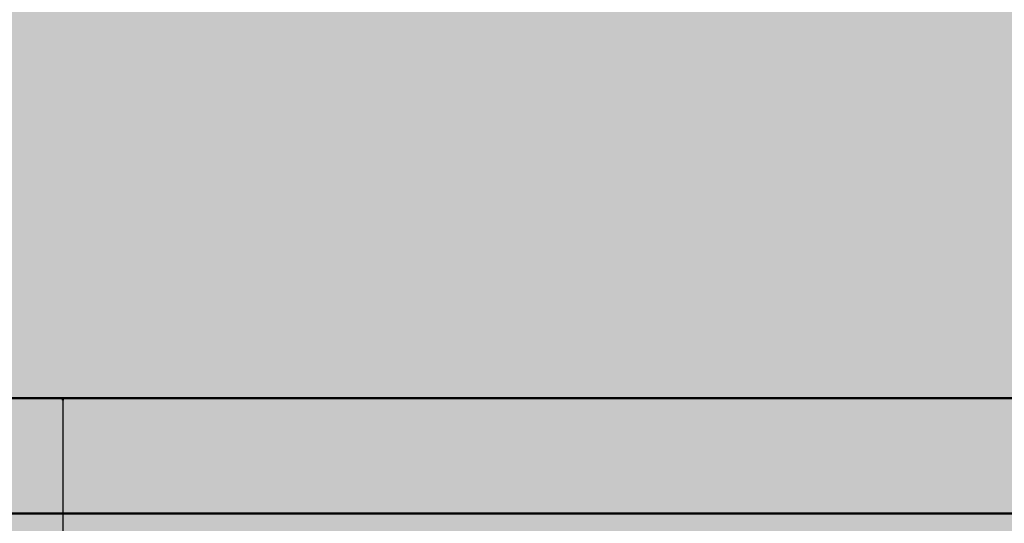
# Model space of a CAD drawing. Units: millimetres. Extents: x 0 to 2267, y 0 to 1823.
# Tile 25 of 256: x 1590 to 1675, y 1117 to 1160. Entities that reach past the tile are written whole.
import ezdxf

# ---------------------------------------------------------------- set-up
doc = ezdxf.new("R2010")
doc.units = ezdxf.units.MM
doc.header["$MEASUREMENT"] = 0
for name, color, linetype, lineweight in [('M-DIMS', 2, 'Continuous', 25), ('M-HATC', 252, 'Continuous', 18), ('M-OUTL', 7, 'Continuous', 50)]:
    doc.layers.add(name, color=color, linetype=linetype, lineweight=lineweight)
doc.styles.get("Standard").update_dxf_attribs({"font": 'arial.ttf'})
doc.dimstyles.get("Standard").update_dxf_attribs({"dimtxt": 7, "dimasz": 4, "dimexe": 0.18, "dimexo": 0.0625, "dimgap": 0.09, "dimtad": 0, "dimdec": 0, "dimzin": 0, "dimdsep": 46, "dimtxsty": 'Standard', "dimcen": 0.09, "dimadec": 0, "dimazin": 0, "dimtfac": 1, "dimtdec": 0, "dimtofl": 0, "dimtmove": 0, "dimatfit": 3, "dimfxl": 1, "dimtolj": 1, "dimtzin": 0, "dimarcsym": 0})

# ---------------------------------------------------------------- blocks, each defined once
blk = doc.blocks.new('*D1')
at = {"layer": 'Defpoints', "color": 0, "transparency": 16777216}
for p in [(1593.429, 1127.417), (1843.429, 1127.417), (1843.429, 955.628)]:
    blk.add_point(p, dxfattribs=at)
at = {"layer": 'M-DIMS', "color": 0, "lineweight": -2, "transparency": 16777216}
for p, q in [((1593.429, 1127.355), (1593.429, 955.448)), ((1843.429, 1127.355), (1843.429, 955.448)), ((1597.429, 955.628), (1710.558, 955.628)), ((1839.429, 955.628), (1726.3, 955.628))]:
    blk.add_line(p, q, dxfattribs=at)
at = {"layer": 'M-DIMS', "color": 0, "transparency": 16777216}
for points in [[(1597.429, 956.294), (1597.429, 954.961), (1593.429, 955.628)], [(1839.429, 956.294), (1839.429, 954.961), (1843.429, 955.628)]]:
    blk.add_solid(points, dxfattribs=at)
at = {"layer": 'M-DIMS', "color": 0, "transparency": 16777216, "insert": (1718.429, 955.628), "char_height": 7, "attachment_point": 5}
blk.add_mtext('\\A1;250', dxfattribs=at)

msp = doc.modelspace()

# ---------------------------------------------------------------- hatches: boundary and pattern name
at = {"layer": 'M-HATC'}
h = msp.add_hatch(color=256, dxfattribs=at)
h.dxf.hatch_style = 1
h.paths.add_polyline_path([(2065.771, 1618.062, 0.236068), (2055.771, 1638.062), (1381.087, 1638.062, 0.236068), (1371.087, 1618.062), (1371.087, 1603.062), (2055.771, 1603.062), (2065.771, 1603.062)])
h.paths.add_polyline_path([(2062.772, 1550.296), (2062.772, 1560.296), (1374.086, 1560.296), (1374.086, 1550.296), (1374.086, 1540.296), (1384.086, 1540.296), (1389.086, 1540.296), (2062.772, 1540.296)])
h.paths.add_polyline_path([(1930.929, 1282.766), (1505.929, 1282.766), (1587.628, 1235.597, 0.131652), (1600.128, 1232.247), (1836.73, 1232.247, 0.131652), (1849.23, 1235.597)])
h.paths.add_polyline_path([(1930.929, 1117.417), (1905.929, 1117.417), (1505.929, 1117.417), (1505.929, 1077.417), (1930.929, 1077.417)])
h = msp.add_hatch(color=256, dxfattribs=at)
h.dxf.hatch_style = 1
h.paths.add_polyline_path([(2055.771, 1603.062), (1381.087, 1603.062), (1381.087, 1598.062), (2055.771, 1598.062)])
h.paths.add_polyline_path([(2055.771, 1598.062), (1381.087, 1598.062), (1381.087, 1593.062), (2055.771, 1593.062)])
h.paths.add_polyline_path([(2051.307, 1536.761), (1385.55, 1536.761), (1385.55, 1526.761), (1387.55, 1526.761), (1388.537, 1525.053), (1385.332, 1521.233), (1385.332, 1521.223), (2050.254, 1522.749), (2048.321, 1525.053), (2049.307, 1526.761), (2051.307, 1526.761)])
edge = h.paths.add_edge_path()
edge.add_arc((1847.535, 1379.149), 135, 222.60306, 222.89085, ccw=False)
edge.add_line((1748.166, 1287.766), (1683.092, 1287.766))
edge.add_arc((1583.724, 1379.149), 135, 317.10915, 317.39694, ccw=False)
edge.add_arc((1678.969, 1290.671), 5, 222.89085, 317.10915, ccw=False)
edge.add_arc((1774.213, 1379.149), 135, 222.60306, 222.89085, ccw=False)
edge.add_line((1674.845, 1287.766), (1609.771, 1287.766))
edge.add_arc((1510.403, 1379.149), 135, 317.10915, 317.39694, ccw=False)
edge.add_arc((1605.647, 1290.671), 5, 222.89085, 317.10915, ccw=False)
edge.add_arc((1700.892, 1379.149), 135, 222.60306, 222.89085, ccw=False)
edge.add_line((1601.524, 1287.766), (1536.45, 1287.766))
edge.add_arc((1437.081, 1379.149), 135, 317.10915, 317.39694, ccw=False)
edge.add_arc((1532.326, 1290.671), 5, 222.89085, 317.10915, ccw=False)
edge.add_arc((1627.571, 1379.149), 135, 222.60306, 222.89085, ccw=False)
edge.add_line((1528.203, 1287.766), (1505.929, 1287.766))
edge.add_spline(control_points=[(1505.929, 1287.766), (1504.262, 1287.766), (1504.262, 1282.766), (1505.929, 1282.766)], knot_values=[0, 0, 0, 0, 5, 5, 5, 5], degree=3, periodic=0)
edge.add_line((1505.929, 1282.766), (1930.929, 1282.766))
edge.add_spline(control_points=[(1930.929, 1282.766), (1932.596, 1282.766), (1932.596, 1287.766), (1930.929, 1287.766)], knot_values=[0, 0, 0, 0, 5, 5, 5, 5], degree=3, periodic=0)
edge.add_line((1930.929, 1287.766), (1903.056, 1287.766))
edge.add_arc((1803.688, 1379.149), 135, 317.10915, 317.39694, ccw=False)
edge.add_arc((1898.932, 1290.671), 5, 222.89085, 317.10915, ccw=False)
edge.add_arc((1994.177, 1379.149), 135, 222.60306, 222.89085, ccw=False)
edge.add_line((1894.809, 1287.766), (1829.735, 1287.766))
edge.add_arc((1730.366, 1379.149), 135, 317.10915, 317.39694, ccw=False)
edge.add_arc((1825.611, 1290.671), 5, 222.89085, 317.10915, ccw=False)
edge.add_arc((1920.856, 1379.149), 135, 222.60306, 222.89085, ccw=False)
edge.add_line((1821.487, 1287.766), (1756.413, 1287.766))
edge.add_arc((1657.045, 1379.149), 135, 317.10915, 317.39694, ccw=False)
edge.add_arc((1752.29, 1290.671), 5, 222.89085, 317.10915, ccw=False)
edge = h.paths.add_edge_path()
edge.add_spline(control_points=[(1843.429, 1227.247), (1845.096, 1227.247), (1845.096, 1232.247), (1843.429, 1232.247)], knot_values=[0, 0, 0, 0, 5, 5, 5, 5], degree=3, periodic=0)
edge.add_line((1843.429, 1232.247), (1593.429, 1232.247))
edge.add_spline(control_points=[(1593.429, 1232.247), (1591.762, 1232.247), (1591.762, 1227.247), (1593.429, 1227.247)], knot_values=[0, 0, 0, 0, 5, 5, 5, 5], degree=3, periodic=0)
edge.add_line((1593.429, 1227.247), (1843.429, 1227.247))
h.paths.add_polyline_path([(1905.929, 1127.417), (1530.929, 1127.417, 0.414214), (1520.929, 1117.417), (1530.929, 1117.417), (1915.929, 1117.417, 0.414214)])
edge = h.paths.add_edge_path()
edge.add_arc((1397.086, 1498.408), 12.73, 90.78215, 190.87871, ccw=False)
edge.add_line((1396.912, 1511.136), (1428.01, 1511.349))
edge.add_line((1428.01, 1511.349), (1433.01, 1511.349))
edge.add_line((1433.01, 1511.349), (1434.439, 1511.349))
edge.add_arc((1419.474, 1498.08), 20, 41.561, 74.08211)
edge.add_line((1424.959, 1517.314), (1399.935, 1517.256))
edge.add_spline(control_points=[(1399.931, 1517.256), (1399.884, 1517.213), (1399.833, 1517.169), (1399.777, 1517.124)], knot_values=[11.567499, 11.567499, 11.567499, 11.567499, 11.814249, 11.814249, 11.814249, 11.814249], degree=3, periodic=0)
edge.add_spline(control_points=[(1399.633, 1517.01), (1399.583, 1516.972), (1399.531, 1516.934), (1399.476, 1516.895)], knot_values=[11.167718, 11.167718, 11.167718, 11.167718, 11.365188, 11.365188, 11.365188, 11.365188], degree=3, periodic=0)
edge.add_spline(control_points=[(1399.34, 1516.8), (1399.151, 1516.672), (1398.938, 1516.538), (1398.704, 1516.399)], knot_values=[10.376405, 10.376405, 10.376405, 10.376405, 11.00994, 11.00994, 11.00994, 11.00994], degree=3, periodic=0)
edge.add_spline(control_points=[(1398.657, 1516.372), (1398.579, 1516.326), (1398.498, 1516.28), (1398.415, 1516.233)], knot_values=[10.125175, 10.125175, 10.125175, 10.125175, 10.334406, 10.334406, 10.334406, 10.334406], degree=3, periodic=0)
edge.add_spline(control_points=[(1398.264, 1516.149), (1398.196, 1516.111), (1398.126, 1516.073), (1398.055, 1516.035)], knot_values=[9.832246, 9.832246, 9.832246, 9.832246, 9.999658, 9.999658, 9.999658, 9.999658], degree=3, periodic=0)
edge.add_spline(control_points=[(1397.999, 1516.005), (1397.731, 1515.862), (1397.446, 1515.717), (1397.147, 1515.571)], knot_values=[9.161808, 9.161808, 9.161808, 9.161808, 9.787769, 9.787769, 9.787769, 9.787769], degree=3, periodic=0)
edge.add_spline(control_points=[(1397.147, 1515.571), (1396.842, 1515.423), (1396.522, 1515.274), (1396.191, 1515.126)], knot_values=[8.524455, 8.524455, 8.524455, 8.524455, 9.161808, 9.161808, 9.161808, 9.161808], degree=3, periodic=0)
edge.add_spline(control_points=[(1396.078, 1515.076), (1395.985, 1515.035), (1395.892, 1514.994), (1395.798, 1514.953)], knot_values=[8.275193, 8.275193, 8.275193, 8.275193, 8.451726, 8.451726, 8.451726, 8.451726], degree=3, periodic=0)
edge.add_spline(control_points=[(1395.602, 1514.869), (1395.5, 1514.826), (1395.397, 1514.782), (1395.293, 1514.739)], knot_values=[7.962917, 7.962917, 7.962917, 7.962917, 8.152764, 8.152764, 8.152764, 8.152764], degree=3, periodic=0)
edge.add_spline(control_points=[(1395.212, 1514.706), (1394.828, 1514.547), (1394.435, 1514.393), (1394.036, 1514.244)], knot_values=[7.21254, 7.21254, 7.21254, 7.21254, 7.913148, 7.913148, 7.913148, 7.913148], degree=3, periodic=0)
edge.add_spline(control_points=[(1394.036, 1514.244), (1393.708, 1514.121), (1393.375, 1514.003), (1393.043, 1513.889)], knot_values=[6.633733, 6.633733, 6.633733, 6.633733, 7.21254, 7.21254, 7.21254, 7.21254], degree=3, periodic=0)
edge.add_spline(control_points=[(1392.821, 1513.815), (1392.72, 1513.781), (1392.618, 1513.748), (1392.517, 1513.715)], knot_values=[6.328796, 6.328796, 6.328796, 6.328796, 6.505493, 6.505493, 6.505493, 6.505493], degree=3, periodic=0)
edge.add_spline(control_points=[(1392.517, 1513.715), (1392.319, 1513.652), (1392.121, 1513.59), (1391.924, 1513.531)], knot_values=[5.984605, 5.984605, 5.984605, 5.984605, 6.328796, 6.328796, 6.328796, 6.328796], degree=3, periodic=0)
edge.add_spline(control_points=[(1391.792, 1513.491), (1391.312, 1513.35), (1390.838, 1513.224), (1390.378, 1513.117)], knot_values=[5.066697, 5.066697, 5.066697, 5.066697, 5.907055, 5.907055, 5.907055, 5.907055], degree=3, periodic=0)
edge.add_spline(control_points=[(1390.378, 1513.117), (1390.18, 1513.071), (1389.984, 1513.028), (1389.791, 1512.99)], knot_values=[4.70367, 4.70367, 4.70367, 4.70367, 5.066695, 5.066695, 5.066695, 5.066695], degree=3, periodic=0)
edge.add_spline(control_points=[(1389.422, 1512.92), (1389.246, 1512.889), (1389.073, 1512.862), (1388.904, 1512.838)], knot_values=[4.130571, 4.130571, 4.130571, 4.130571, 4.469816, 4.469816, 4.469816, 4.469816], degree=3, periodic=0)
edge.add_spline(control_points=[(1388.904, 1512.838), (1388.591, 1512.795), (1388.291, 1512.764), (1388.007, 1512.749)], knot_values=[3.504031, 3.504031, 3.504031, 3.504031, 4.130571, 4.130571, 4.130571, 4.130571], degree=3, periodic=0)
edge.add_spline(control_points=[(1387.936, 1512.746), (1387.854, 1512.742), (1387.773, 1512.74), (1387.694, 1512.739)], knot_values=[3.268866, 3.268866, 3.268866, 3.268866, 3.451164, 3.451164, 3.451164, 3.451164], degree=3, periodic=0)
edge.add_spline(control_points=[(1387.335, 1512.744), (1387.208, 1512.75), (1387.085, 1512.76), (1386.967, 1512.774)], knot_values=[2.670686, 2.670686, 2.670686, 2.670686, 2.984, 2.984, 2.984, 2.984], degree=3, periodic=0)
edge.add_spline(control_points=[(1386.833, 1512.792), (1386.821, 1512.794), (1386.809, 1512.796), (1386.797, 1512.798)], knot_values=[2.516981, 2.516981, 2.516981, 2.516981, 2.549528, 2.549528, 2.549528, 2.549528], degree=3, periodic=0)
edge.add_spline(control_points=[(1386.453, 1512.873), (1386.426, 1512.881), (1386.399, 1512.889), (1386.373, 1512.897)], knot_values=[2.095869, 2.095869, 2.095869, 2.095869, 2.17941, 2.17941, 2.17941, 2.17941], degree=3, periodic=0)
edge.add_spline(control_points=[(1386.069, 1513.019), (1386.063, 1513.022), (1386.058, 1513.025), (1386.052, 1513.028)], knot_values=[1.72453, 1.72453, 1.72453, 1.72453, 1.745933, 1.745933, 1.745933, 1.745933], degree=3, periodic=0)
edge.add_arc((1399.474, 1498.08), 20, 131.82432, 180)
edge.add_arc((1630.334, 1505.548), 250.971, 181.70518, 236.42798)
edge.add_arc((1605.34, 1483.304), 218.782, 238.66083, 243.34961)
edge.add_arc((1647.091, 1510.359), 262.899, 183.12984, 237.85344, ccw=False)
h.paths.add_polyline_path([(1406.537, 1391.964, 0.149382), (1491.551, 1296.442, -0.129517)], flags=17)
edge = h.paths.add_edge_path()
edge.add_arc((2037.384, 1498.08), 20, 0, 48.26587)
edge.add_spline(control_points=[(2050.697, 1513.005), (2050.651, 1512.985), (2050.603, 1512.966), (2050.554, 1512.948)], knot_values=[1.835652, 1.835652, 1.835652, 1.835652, 2.000781, 2.000781, 2.000781, 2.000781], degree=3, periodic=0)
edge.add_spline(control_points=[(2050.462, 1512.917), (2050.479, 1512.922), (2050.496, 1512.928), (2050.513, 1512.934)], knot_values=[2.045477, 2.045477, 2.045477, 2.045477, 2.101389, 2.101389, 2.101389, 2.101389], degree=3, periodic=0)
edge.add_spline(control_points=[(2050.129, 1512.834), (2050.198, 1512.847), (2050.266, 1512.862), (2050.331, 1512.879)], knot_values=[2.237629, 2.237629, 2.237629, 2.237629, 2.435841, 2.435841, 2.435841, 2.435841], degree=3, periodic=0)
edge.add_spline(control_points=[(2050.095, 1512.828), (2050.106, 1512.83), (2050.118, 1512.832), (2050.129, 1512.834)], knot_values=[2.435841, 2.435841, 2.435841, 2.435841, 2.468321, 2.468321, 2.468321, 2.468321], degree=3, periodic=0)
edge.add_spline(control_points=[(2049.784, 1512.785), (2049.855, 1512.792), (2049.924, 1512.801), (2049.992, 1512.811)], knot_values=[2.563852, 2.563852, 2.563852, 2.563852, 2.748541, 2.748541, 2.748541, 2.748541], degree=3, periodic=0)
edge.add_spline(control_points=[(2049.405, 1512.762), (2049.536, 1512.765), (2049.663, 1512.773), (2049.784, 1512.785)], knot_values=[2.748541, 2.748541, 2.748541, 2.748541, 3.064882, 3.064882, 3.064882, 3.064882], degree=3, periodic=0)
edge.add_spline(control_points=[(2049.17, 1512.76), (2049.234, 1512.759), (2049.297, 1512.759), (2049.358, 1512.761)], knot_values=[3.102309, 3.102309, 3.102309, 3.102309, 3.2503, 3.2503, 3.2503, 3.2503], degree=3, periodic=0)
edge.add_spline(control_points=[(2048.857, 1512.769), (2048.964, 1512.764), (2049.068, 1512.761), (2049.17, 1512.76)], knot_values=[3.2503, 3.2503, 3.2503, 3.2503, 3.486069, 3.486069, 3.486069, 3.486069], degree=3, periodic=0)
edge.add_spline(control_points=[(2048.692, 1512.779), (2048.373, 1512.801), (2048.035, 1512.841), (2047.682, 1512.897)], knot_values=[3.606429, 3.606429, 3.606429, 3.606429, 4.2989, 4.2989, 4.2989, 4.2989], degree=3, periodic=0)
edge.add_spline(control_points=[(2047.682, 1512.897), (2047.546, 1512.919), (2047.408, 1512.942), (2047.268, 1512.969)], knot_values=[4.2989, 4.2989, 4.2989, 4.2989, 4.565769, 4.565769, 4.565769, 4.565769], degree=3, periodic=0)
edge.add_spline(control_points=[(2047.268, 1512.969), (2047.145, 1512.991), (2047.021, 1513.016), (2046.895, 1513.042)], knot_values=[4.565769, 4.565769, 4.565769, 4.565769, 4.799971, 4.799971, 4.799971, 4.799971], degree=3, periodic=0)
edge.add_spline(control_points=[(2046.895, 1513.042), (2046.529, 1513.119), (2046.151, 1513.209), (2045.768, 1513.311)], knot_values=[4.799971, 4.799971, 4.799971, 4.799971, 5.483718, 5.483718, 5.483718, 5.483718], degree=3, periodic=0)
edge.add_spline(control_points=[(2045.768, 1513.311), (2045.372, 1513.415), (2044.97, 1513.532), (2044.566, 1513.659)], knot_values=[5.483718, 5.483718, 5.483718, 5.483718, 6.187866, 6.187866, 6.187866, 6.187866], degree=3, periodic=0)
edge.add_spline(control_points=[(2044.566, 1513.659), (2044.415, 1513.706), (2044.263, 1513.755), (2044.112, 1513.805)], knot_values=[6.187866, 6.187866, 6.187866, 6.187866, 6.451551, 6.451551, 6.451551, 6.451551], degree=3, periodic=0)
edge.add_spline(control_points=[(2044.112, 1513.805), (2043.997, 1513.843), (2043.882, 1513.881), (2043.767, 1513.92)], knot_values=[6.451551, 6.451551, 6.451551, 6.451551, 6.651434, 6.651434, 6.651434, 6.651434], degree=3, periodic=0)
edge.add_spline(control_points=[(2043.767, 1513.92), (2043.372, 1514.055), (2042.977, 1514.198), (2042.589, 1514.346)], knot_values=[6.651434, 6.651434, 6.651434, 6.651434, 7.338879, 7.338879, 7.338879, 7.338879], degree=3, periodic=0)
edge.add_spline(control_points=[(2042.589, 1514.346), (2042.164, 1514.507), (2041.746, 1514.675), (2041.341, 1514.846)], knot_values=[7.338879, 7.338879, 7.338879, 7.338879, 8.089209, 8.089209, 8.089209, 8.089209], degree=3, periodic=0)
edge.add_spline(control_points=[(2041.341, 1514.846), (2041.103, 1514.946), (2040.869, 1515.048), (2040.64, 1515.15)], knot_values=[8.089209, 8.089209, 8.089209, 8.089209, 8.529587, 8.529587, 8.529587, 8.529587], degree=3, periodic=0)
edge.add_spline(control_points=[(2040.51, 1515.209), (2040.082, 1515.402), (2039.675, 1515.597), (2039.295, 1515.789)], knot_values=[8.613818, 8.613818, 8.613818, 8.613818, 9.44571, 9.44571, 9.44571, 9.44571], degree=3, periodic=0)
edge.add_spline(control_points=[(2039.295, 1515.789), (2039.062, 1515.907), (2038.839, 1516.025), (2038.629, 1516.14)], knot_values=[9.44571, 9.44571, 9.44571, 9.44571, 9.956404, 9.956404, 9.956404, 9.956404], degree=3, periodic=0)
edge.add_spline(control_points=[(2038.629, 1516.14), (2038.519, 1516.2), (2038.412, 1516.26), (2038.309, 1516.319)], knot_values=[9.956404, 9.956404, 9.956404, 9.956404, 10.223542, 10.223542, 10.223542, 10.223542], degree=3, periodic=0)
edge.add_spline(control_points=[(2038.309, 1516.319), (2038.214, 1516.374), (2038.122, 1516.428), (2038.033, 1516.481)], knot_values=[10.223542, 10.223542, 10.223542, 10.223542, 10.47051, 10.47051, 10.47051, 10.47051], degree=3, periodic=0)
edge.add_spline(control_points=[(2038.033, 1516.481), (2037.786, 1516.63), (2037.564, 1516.773), (2037.372, 1516.909)], knot_values=[10.47051, 10.47051, 10.47051, 10.47051, 11.15767, 11.15767, 11.15767, 11.15767], degree=3, periodic=0)
edge.add_spline(control_points=[(2037.372, 1516.909), (2037.279, 1516.975), (2037.193, 1517.04), (2037.114, 1517.102)], knot_values=[11.15767, 11.15767, 11.15767, 11.15767, 11.49227, 11.49227, 11.49227, 11.49227], degree=3, periodic=0)
edge.add_spline(control_points=[(2036.856, 1517.326), (2036.915, 1517.269), (2036.981, 1517.21), (2037.056, 1517.149)], knot_values=[11.577341, 11.577341, 11.577341, 11.577341, 11.91035, 11.91035, 11.91035, 11.91035], degree=3, periodic=0)
edge.add_spline(control_points=[(2036.807, 1517.375), (2036.823, 1517.359), (2036.839, 1517.342), (2036.856, 1517.326)], knot_values=[11.91035, 11.91035, 11.91035, 11.91035, 12.007402, 12.007402, 12.007402, 12.007402], degree=3, periodic=0)
edge.add_spline(control_points=[(2036.702, 1517.494), (2036.71, 1517.483), (2036.72, 1517.472), (2036.729, 1517.461)], knot_values=[12.184155, 12.184155, 12.184155, 12.184155, 12.255409, 12.255409, 12.255409, 12.255409], degree=3, periodic=0)
edge.add_spline(control_points=[(2036.616, 1517.621), (2036.62, 1517.613), (2036.624, 1517.606), (2036.629, 1517.598)], knot_values=[12.487913, 12.487913, 12.487913, 12.487913, 12.541035, 12.541035, 12.541035, 12.541035], degree=3, periodic=0)
edge.add_spline(control_points=[(2036.563, 1517.786), (2036.564, 1517.779), (2036.564, 1517.773), (2036.565, 1517.766)], knot_values=[12.911761, 12.911761, 12.911761, 12.911761, 12.968286, 12.968286, 12.968286, 12.968286], degree=3, periodic=0)
edge.add_spline(control_points=[(2036.617, 1517.93), (2036.612, 1517.926), (2036.609, 1517.921), (2036.605, 1517.916)], knot_values=[13.382527, 13.382527, 13.382527, 13.382527, 13.433791, 13.433791, 13.433791, 13.433791], degree=3, periodic=0)
edge.add_spline(control_points=[(2036.749, 1518.017), (2036.736, 1518.012), (2036.724, 1518.006), (2036.712, 1518)], knot_values=[13.726299, 13.726299, 13.726299, 13.726299, 13.809928, 13.809928, 13.809928, 13.809928], degree=3, periodic=0)
edge.add_spline(control_points=[(2036.86, 1518.053), (2036.839, 1518.047), (2036.818, 1518.042), (2036.799, 1518.035)], knot_values=[13.910887, 13.910887, 13.910887, 13.910887, 14.02153, 14.02153, 14.02153, 14.02153], degree=3, periodic=0)
edge.add_line((2036.964, 1518.08), (2032.384, 1518.08))
edge.add_line((2032.384, 1518.08), (2027.384, 1518.08))
edge.add_line((2027.384, 1518.08), (2022.384, 1518.08))
edge.add_line((2022.384, 1518.08), (2017.384, 1518.08))
edge.add_arc((2017.384, 1498.08), 20, 90, 138.439)
edge.add_line((2002.419, 1511.349), (2003.848, 1511.349))
edge.add_line((2003.848, 1511.349), (2008.848, 1511.349))
edge.add_line((2008.848, 1511.349), (2039.772, 1511.138))
edge.add_arc((2039.772, 1498.408), 12.73, -10.87871, 90, ccw=False)
edge.add_arc((1789.767, 1510.359), 262.899, 302.14656, 356.87016, ccw=False)
edge.add_arc((1831.518, 1483.304), 218.782, 296.65039, 301.33917)
edge.add_arc((1806.524, 1505.548), 250.971, 303.57202, 358.29482)
h.paths.add_polyline_path([(2030.321, 1391.964, -0.129517), (1945.307, 1296.442, 0.149382)], flags=17)
edge = h.paths.add_edge_path()
edge.add_spline(control_points=[(2037.246, 1518.082), (2037.29, 1518.081), (2037.336, 1518.08), (2037.384, 1518.08)], knot_values=[0.000012, 0.000012, 0.000012, 0.000012, 0.144754, 0.144754, 0.144754, 0.144754], degree=3, periodic=0)
edge.add_line((2037.336, 1518.08), (2037.01, 1518.08))
edge.add_spline(control_points=[(2037.01, 1518.08), (2036.982, 1518.077), (2036.956, 1518.073), (2036.931, 1518.068)], knot_values=[14.13465, 14.13465, 14.13465, 14.13465, 14.247197, 14.247197, 14.247197, 14.247197], degree=3, periodic=0)
edge.add_spline(control_points=[(2036.931, 1518.068), (2036.928, 1518.067), (2036.924, 1518.067), (2036.921, 1518.066)], knot_values=[14.118315, 14.118315, 14.118315, 14.118315, 14.13465, 14.13465, 14.13465, 14.13465], degree=3, periodic=0)
edge.add_spline(control_points=[(2036.921, 1518.066), (2036.912, 1518.064), (2036.903, 1518.063), (2036.895, 1518.061)], knot_values=[14.078086, 14.078086, 14.078086, 14.078086, 14.118315, 14.118315, 14.118315, 14.118315], degree=3, periodic=0)
edge.add_spline(control_points=[(2036.895, 1518.061), (2036.883, 1518.058), (2036.872, 1518.056), (2036.86, 1518.053)], knot_values=[14.02153, 14.02153, 14.02153, 14.02153, 14.078086, 14.078086, 14.078086, 14.078086], degree=3, periodic=0)
edge.add_spline(control_points=[(2036.86, 1518.053), (2036.839, 1518.047), (2036.818, 1518.042), (2036.799, 1518.035)], knot_values=[13.910887, 13.910887, 13.910887, 13.910887, 14.02153, 14.02153, 14.02153, 14.02153], degree=3, periodic=0)
edge.add_spline(control_points=[(2036.799, 1518.035), (2036.798, 1518.035), (2036.797, 1518.035), (2036.797, 1518.035)], knot_values=[13.906906, 13.906906, 13.906906, 13.906906, 13.910887, 13.910887, 13.910887, 13.910887], degree=3, periodic=0)
edge.add_spline(control_points=[(2036.797, 1518.035), (2036.788, 1518.032), (2036.78, 1518.029), (2036.772, 1518.026)], knot_values=[13.857826, 13.857826, 13.857826, 13.857826, 13.906906, 13.906906, 13.906906, 13.906906], degree=3, periodic=0)
edge.add_spline(control_points=[(2036.772, 1518.026), (2036.764, 1518.023), (2036.756, 1518.02), (2036.749, 1518.017)], knot_values=[13.809928, 13.809928, 13.809928, 13.809928, 13.857826, 13.857826, 13.857826, 13.857826], degree=3, periodic=0)
edge.add_spline(control_points=[(2036.749, 1518.017), (2036.736, 1518.012), (2036.724, 1518.006), (2036.712, 1518)], knot_values=[13.726299, 13.726299, 13.726299, 13.726299, 13.809928, 13.809928, 13.809928, 13.809928], degree=3, periodic=0)
edge.add_spline(control_points=[(2036.712, 1518), (2036.712, 1518), (2036.712, 1518), (2036.711, 1518)], knot_values=[13.723993, 13.723993, 13.723993, 13.723993, 13.726299, 13.726299, 13.726299, 13.726299], degree=3, periodic=0)
edge.add_spline(control_points=[(2036.711, 1518), (2036.706, 1517.997), (2036.701, 1517.994), (2036.696, 1517.992)], knot_values=[13.686536, 13.686536, 13.686536, 13.686536, 13.723993, 13.723993, 13.723993, 13.723993], degree=3, periodic=0)
edge.add_spline(control_points=[(2036.696, 1517.992), (2036.692, 1517.989), (2036.687, 1517.987), (2036.683, 1517.984)], knot_values=[13.651251, 13.651251, 13.651251, 13.651251, 13.686536, 13.686536, 13.686536, 13.686536], degree=3, periodic=0)
edge.add_spline(control_points=[(2036.683, 1517.984), (2036.676, 1517.98), (2036.67, 1517.976), (2036.664, 1517.971)], knot_values=[13.596804, 13.596804, 13.596804, 13.596804, 13.651251, 13.651251, 13.651251, 13.651251], degree=3, periodic=0)
edge.add_spline(control_points=[(2036.664, 1517.971), (2036.664, 1517.971), (2036.663, 1517.971), (2036.663, 1517.971)], knot_values=[13.593956, 13.593956, 13.593956, 13.593956, 13.596804, 13.596804, 13.596804, 13.596804], degree=3, periodic=0)
edge.add_spline(control_points=[(2036.663, 1517.971), (2036.66, 1517.969), (2036.658, 1517.967), (2036.655, 1517.965)], knot_values=[13.570322, 13.570322, 13.570322, 13.570322, 13.593956, 13.593956, 13.593956, 13.593956], degree=3, periodic=0)
edge.add_spline(control_points=[(2036.655, 1517.965), (2036.653, 1517.963), (2036.65, 1517.961), (2036.647, 1517.959)], knot_values=[13.545477, 13.545477, 13.545477, 13.545477, 13.570322, 13.570322, 13.570322, 13.570322], degree=3, periodic=0)
edge.add_spline(control_points=[(2036.647, 1517.959), (2036.647, 1517.959), (2036.647, 1517.959), (2036.647, 1517.959)], knot_values=[13.543931, 13.543931, 13.543931, 13.543931, 13.545477, 13.545477, 13.545477, 13.545477], degree=3, periodic=0)
edge.add_spline(control_points=[(2036.647, 1517.959), (2036.641, 1517.954), (2036.636, 1517.949), (2036.631, 1517.945)], knot_values=[13.488237, 13.488237, 13.488237, 13.488237, 13.543931, 13.543931, 13.543931, 13.543931], degree=3, periodic=0)
edge.add_spline(control_points=[(2036.631, 1517.945), (2036.628, 1517.942), (2036.626, 1517.94), (2036.623, 1517.937)], knot_values=[13.460307, 13.460307, 13.460307, 13.460307, 13.488237, 13.488237, 13.488237, 13.488237], degree=3, periodic=0)
edge.add_spline(control_points=[(2036.623, 1517.937), (2036.622, 1517.936), (2036.62, 1517.934), (2036.618, 1517.932)], knot_values=[13.439712, 13.439712, 13.439712, 13.439712, 13.460307, 13.460307, 13.460307, 13.460307], degree=3, periodic=0)
edge.add_spline(control_points=[(2036.618, 1517.932), (2036.618, 1517.931), (2036.617, 1517.931), (2036.617, 1517.93)], knot_values=[13.433791, 13.433791, 13.433791, 13.433791, 13.439712, 13.439712, 13.439712, 13.439712], degree=3, periodic=0)
edge.add_spline(control_points=[(2036.617, 1517.93), (2036.612, 1517.926), (2036.609, 1517.921), (2036.605, 1517.916)], knot_values=[13.382527, 13.382527, 13.382527, 13.382527, 13.433791, 13.433791, 13.433791, 13.433791], degree=3, periodic=0)
edge.add_spline(control_points=[(2036.605, 1517.916), (2036.603, 1517.913), (2036.6, 1517.91), (2036.598, 1517.907)], knot_values=[13.350017, 13.350017, 13.350017, 13.350017, 13.382527, 13.382527, 13.382527, 13.382527], degree=3, periodic=0)
edge.add_spline(control_points=[(2036.598, 1517.907), (2036.597, 1517.906), (2036.596, 1517.904), (2036.595, 1517.903)], knot_values=[13.333922, 13.333922, 13.333922, 13.333922, 13.350017, 13.350017, 13.350017, 13.350017], degree=3, periodic=0)
edge.add_spline(control_points=[(2036.595, 1517.903), (2036.595, 1517.902), (2036.594, 1517.901), (2036.593, 1517.9)], knot_values=[13.323828, 13.323828, 13.323828, 13.323828, 13.333922, 13.333922, 13.333922, 13.333922], degree=3, periodic=0)
edge.add_spline(control_points=[(2036.593, 1517.9), (2036.59, 1517.895), (2036.588, 1517.891), (2036.585, 1517.886)], knot_values=[13.277545, 13.277545, 13.277545, 13.277545, 13.323828, 13.323828, 13.323828, 13.323828], degree=3, periodic=0)
edge.add_spline(control_points=[(2036.585, 1517.886), (2036.584, 1517.883), (2036.582, 1517.879), (2036.58, 1517.875)], knot_values=[13.240119, 13.240119, 13.240119, 13.240119, 13.277545, 13.277545, 13.277545, 13.277545], degree=3, periodic=0)
edge.add_spline(control_points=[(2036.58, 1517.875), (2036.58, 1517.874), (2036.579, 1517.873), (2036.578, 1517.872)], knot_values=[13.228211, 13.228211, 13.228211, 13.228211, 13.240119, 13.240119, 13.240119, 13.240119], degree=3, periodic=0)
edge.add_spline(control_points=[(2036.578, 1517.872), (2036.578, 1517.87), (2036.577, 1517.869), (2036.577, 1517.868)], knot_values=[13.215717, 13.215717, 13.215717, 13.215717, 13.228211, 13.228211, 13.228211, 13.228211], degree=3, periodic=0)
edge.add_spline(control_points=[(2036.577, 1517.868), (2036.575, 1517.864), (2036.574, 1517.86), (2036.573, 1517.857)], knot_values=[13.179847, 13.179847, 13.179847, 13.179847, 13.215717, 13.215717, 13.215717, 13.215717], degree=3, periodic=0)
edge.add_spline(control_points=[(2036.573, 1517.857), (2036.571, 1517.851), (2036.57, 1517.846), (2036.569, 1517.841)], knot_values=[13.132017, 13.132017, 13.132017, 13.132017, 13.179847, 13.179847, 13.179847, 13.179847], degree=3, periodic=0)
edge.add_spline(control_points=[(2036.569, 1517.841), (2036.568, 1517.84), (2036.568, 1517.839), (2036.568, 1517.838)], knot_values=[13.122482, 13.122482, 13.122482, 13.122482, 13.132017, 13.132017, 13.132017, 13.132017], degree=3, periodic=0)
edge.add_spline(control_points=[(2036.568, 1517.838), (2036.568, 1517.836), (2036.567, 1517.835), (2036.567, 1517.833)], knot_values=[13.105592, 13.105592, 13.105592, 13.105592, 13.122482, 13.122482, 13.122482, 13.122482], degree=3, periodic=0)
edge.add_spline(control_points=[(2036.567, 1517.833), (2036.566, 1517.829), (2036.566, 1517.826), (2036.565, 1517.822)], knot_values=[13.074063, 13.074063, 13.074063, 13.074063, 13.105592, 13.105592, 13.105592, 13.105592], degree=3, periodic=0)
edge.add_spline(control_points=[(2036.565, 1517.822), (2036.565, 1517.822), (2036.565, 1517.822), (2036.565, 1517.822)], knot_values=[13.074043, 13.074043, 13.074043, 13.074043, 13.074063, 13.074063, 13.074063, 13.074063], degree=3, periodic=0)
edge.add_spline(control_points=[(2036.565, 1517.822), (2036.564, 1517.816), (2036.564, 1517.811), (2036.564, 1517.805)], knot_values=[13.021884, 13.021884, 13.021884, 13.021884, 13.074043, 13.074043, 13.074043, 13.074043], degree=3, periodic=0)
edge.add_spline(control_points=[(2036.564, 1517.805), (2036.564, 1517.804), (2036.564, 1517.803), (2036.564, 1517.803)], knot_values=[13.01674, 13.01674, 13.01674, 13.01674, 13.021884, 13.021884, 13.021884, 13.021884], degree=3, periodic=0)
edge.add_spline(control_points=[(2036.564, 1517.803), (2036.563, 1517.801), (2036.563, 1517.798), (2036.563, 1517.796)], knot_values=[12.996438, 12.996438, 12.996438, 12.996438, 13.01674, 13.01674, 13.01674, 13.01674], degree=3, periodic=0)
edge.add_spline(control_points=[(2036.563, 1517.796), (2036.563, 1517.793), (2036.563, 1517.789), (2036.563, 1517.786)], knot_values=[12.968286, 12.968286, 12.968286, 12.968286, 12.996438, 12.996438, 12.996438, 12.996438], degree=3, periodic=0)
edge.add_spline(control_points=[(2036.563, 1517.786), (2036.564, 1517.779), (2036.564, 1517.773), (2036.565, 1517.766)], knot_values=[12.911761, 12.911761, 12.911761, 12.911761, 12.968286, 12.968286, 12.968286, 12.968286], degree=3, periodic=0)
edge.add_spline(control_points=[(2036.565, 1517.766), (2036.565, 1517.766), (2036.565, 1517.766), (2036.565, 1517.766)], knot_values=[12.911017, 12.911017, 12.911017, 12.911017, 12.911761, 12.911761, 12.911761, 12.911761], degree=3, periodic=0)
edge.add_spline(control_points=[(2036.565, 1517.766), (2036.565, 1517.762), (2036.566, 1517.759), (2036.566, 1517.756)], knot_values=[12.88528, 12.88528, 12.88528, 12.88528, 12.911017, 12.911017, 12.911017, 12.911017], degree=3, periodic=0)
edge.add_spline(control_points=[(2036.566, 1517.756), (2036.567, 1517.753), (2036.567, 1517.751), (2036.568, 1517.748)], knot_values=[12.862519, 12.862519, 12.862519, 12.862519, 12.88528, 12.88528, 12.88528, 12.88528], degree=3, periodic=0)
edge.add_spline(control_points=[(2036.568, 1517.748), (2036.568, 1517.747), (2036.568, 1517.747), (2036.568, 1517.746)], knot_values=[12.858885, 12.858885, 12.858885, 12.858885, 12.862519, 12.862519, 12.862519, 12.862519], degree=3, periodic=0)
edge.add_spline(control_points=[(2036.568, 1517.746), (2036.569, 1517.74), (2036.571, 1517.733), (2036.572, 1517.726)], knot_values=[12.8053, 12.8053, 12.8053, 12.8053, 12.858885, 12.858885, 12.858885, 12.858885], degree=3, periodic=0)
edge.add_spline(control_points=[(2036.572, 1517.726), (2036.573, 1517.723), (2036.574, 1517.719), (2036.576, 1517.715)], knot_values=[12.775176, 12.775176, 12.775176, 12.775176, 12.8053, 12.8053, 12.8053, 12.8053], degree=3, periodic=0)
edge.add_spline(control_points=[(2036.576, 1517.715), (2036.576, 1517.713), (2036.577, 1517.71), (2036.578, 1517.708)], knot_values=[12.756759, 12.756759, 12.756759, 12.756759, 12.775176, 12.775176, 12.775176, 12.775176], degree=3, periodic=0)
edge.add_spline(control_points=[(2036.578, 1517.708), (2036.578, 1517.707), (2036.578, 1517.706), (2036.579, 1517.705)], knot_values=[12.748742, 12.748742, 12.748742, 12.748742, 12.756759, 12.756759, 12.756759, 12.756759], degree=3, periodic=0)
edge.add_spline(control_points=[(2036.579, 1517.705), (2036.581, 1517.698), (2036.583, 1517.692), (2036.586, 1517.685)], knot_values=[12.69959, 12.69959, 12.69959, 12.69959, 12.748742, 12.748742, 12.748742, 12.748742], degree=3, periodic=0)
edge.add_spline(control_points=[(2036.586, 1517.685), (2036.588, 1517.68), (2036.59, 1517.675), (2036.592, 1517.669)], knot_values=[12.659038, 12.659038, 12.659038, 12.659038, 12.69959, 12.69959, 12.69959, 12.69959], degree=3, periodic=0)
edge.add_spline(control_points=[(2036.592, 1517.669), (2036.594, 1517.665), (2036.596, 1517.66), (2036.598, 1517.656)], knot_values=[12.626806, 12.626806, 12.626806, 12.626806, 12.659038, 12.659038, 12.659038, 12.659038], degree=3, periodic=0)
edge.add_spline(control_points=[(2036.598, 1517.656), (2036.598, 1517.655), (2036.599, 1517.654), (2036.599, 1517.653)], knot_values=[12.619394, 12.619394, 12.619394, 12.619394, 12.626806, 12.626806, 12.626806, 12.626806], degree=3, periodic=0)
edge.add_spline(control_points=[(2036.599, 1517.653), (2036.604, 1517.642), (2036.61, 1517.632), (2036.616, 1517.621)], knot_values=[12.541039, 12.541039, 12.541039, 12.541039, 12.619394, 12.619394, 12.619394, 12.619394], degree=3, periodic=0)
edge.add_spline(control_points=[(2036.616, 1517.621), (2036.616, 1517.621), (2036.616, 1517.621), (2036.616, 1517.621)], knot_values=[12.541035, 12.541035, 12.541035, 12.541035, 12.541039, 12.541039, 12.541039, 12.541039], degree=3, periodic=0)
edge.add_spline(control_points=[(2036.616, 1517.621), (2036.62, 1517.613), (2036.624, 1517.606), (2036.629, 1517.598)], knot_values=[12.487913, 12.487913, 12.487913, 12.487913, 12.541035, 12.541035, 12.541035, 12.541035], degree=3, periodic=0)
edge.add_spline(control_points=[(2036.629, 1517.598), (2036.633, 1517.592), (2036.637, 1517.585), (2036.641, 1517.579)], knot_values=[12.443982, 12.443982, 12.443982, 12.443982, 12.487913, 12.487913, 12.487913, 12.487913], degree=3, periodic=0)
edge.add_spline(control_points=[(2036.641, 1517.579), (2036.641, 1517.578), (2036.642, 1517.576), (2036.643, 1517.575)], knot_values=[12.434996, 12.434996, 12.434996, 12.434996, 12.443982, 12.443982, 12.443982, 12.443982], degree=3, periodic=0)
edge.add_spline(control_points=[(2036.643, 1517.575), (2036.653, 1517.56), (2036.664, 1517.544), (2036.676, 1517.528)], knot_values=[12.329647, 12.329647, 12.329647, 12.329647, 12.434996, 12.434996, 12.434996, 12.434996], degree=3, periodic=0)
edge.add_spline(control_points=[(2036.676, 1517.528), (2036.684, 1517.517), (2036.693, 1517.505), (2036.702, 1517.494)], knot_values=[12.255409, 12.255409, 12.255409, 12.255409, 12.329647, 12.329647, 12.329647, 12.329647], degree=3, periodic=0)
edge.add_spline(control_points=[(2036.702, 1517.494), (2036.71, 1517.483), (2036.72, 1517.472), (2036.729, 1517.461)], knot_values=[12.184155, 12.184155, 12.184155, 12.184155, 12.255409, 12.255409, 12.255409, 12.255409], degree=3, periodic=0)
edge.add_spline(control_points=[(2036.729, 1517.461), (2036.744, 1517.444), (2036.759, 1517.426), (2036.775, 1517.409)], knot_values=[12.075961, 12.075961, 12.075961, 12.075961, 12.184155, 12.184155, 12.184155, 12.184155], degree=3, periodic=0)
edge.add_spline(control_points=[(2036.775, 1517.409), (2036.776, 1517.407), (2036.777, 1517.406), (2036.778, 1517.405)], knot_values=[12.069502, 12.069502, 12.069502, 12.069502, 12.075961, 12.075961, 12.075961, 12.075961], degree=3, periodic=0)
edge.add_spline(control_points=[(2036.778, 1517.405), (2036.788, 1517.395), (2036.797, 1517.385), (2036.807, 1517.375)], knot_values=[12.007402, 12.007402, 12.007402, 12.007402, 12.069502, 12.069502, 12.069502, 12.069502], degree=3, periodic=0)
edge.add_spline(control_points=[(2036.807, 1517.375), (2036.823, 1517.359), (2036.839, 1517.342), (2036.856, 1517.326)], knot_values=[11.91035, 11.91035, 11.91035, 11.91035, 12.007402, 12.007402, 12.007402, 12.007402], degree=3, periodic=0)
edge.add_spline(control_points=[(2036.856, 1517.326), (2036.915, 1517.269), (2036.981, 1517.21), (2037.056, 1517.149)], knot_values=[11.577341, 11.577341, 11.577341, 11.577341, 11.91035, 11.91035, 11.91035, 11.91035], degree=3, periodic=0)
edge.add_spline(control_points=[(2037.056, 1517.149), (2037.075, 1517.134), (2037.094, 1517.118), (2037.114, 1517.102)], knot_values=[11.49227, 11.49227, 11.49227, 11.49227, 11.577341, 11.577341, 11.577341, 11.577341], degree=3, periodic=0)
edge.add_spline(control_points=[(2037.114, 1517.102), (2037.193, 1517.04), (2037.279, 1516.975), (2037.372, 1516.909)], knot_values=[11.15767, 11.15767, 11.15767, 11.15767, 11.49227, 11.49227, 11.49227, 11.49227], degree=3, periodic=0)
edge.add_spline(control_points=[(2037.372, 1516.909), (2037.564, 1516.773), (2037.786, 1516.63), (2038.033, 1516.481)], knot_values=[10.47051, 10.47051, 10.47051, 10.47051, 11.15767, 11.15767, 11.15767, 11.15767], degree=3, periodic=0)
edge.add_spline(control_points=[(2038.033, 1516.481), (2038.122, 1516.428), (2038.214, 1516.374), (2038.309, 1516.319)], knot_values=[10.223542, 10.223542, 10.223542, 10.223542, 10.47051, 10.47051, 10.47051, 10.47051], degree=3, periodic=0)
edge.add_spline(control_points=[(2038.309, 1516.319), (2038.412, 1516.26), (2038.519, 1516.2), (2038.629, 1516.14)], knot_values=[9.956404, 9.956404, 9.956404, 9.956404, 10.223542, 10.223542, 10.223542, 10.223542], degree=3, periodic=0)
edge.add_spline(control_points=[(2038.629, 1516.14), (2038.839, 1516.025), (2039.062, 1515.907), (2039.295, 1515.789)], knot_values=[9.44571, 9.44571, 9.44571, 9.44571, 9.956404, 9.956404, 9.956404, 9.956404], degree=3, periodic=0)
edge.add_spline(control_points=[(2039.295, 1515.789), (2039.675, 1515.597), (2040.082, 1515.402), (2040.51, 1515.209)], knot_values=[8.613818, 8.613818, 8.613818, 8.613818, 9.44571, 9.44571, 9.44571, 9.44571], degree=3, periodic=0)
edge.add_spline(control_points=[(2040.51, 1515.209), (2040.553, 1515.189), (2040.597, 1515.17), (2040.64, 1515.15)], knot_values=[8.529587, 8.529587, 8.529587, 8.529587, 8.613818, 8.613818, 8.613818, 8.613818], degree=3, periodic=0)
edge.add_spline(control_points=[(2040.64, 1515.15), (2040.869, 1515.048), (2041.103, 1514.946), (2041.341, 1514.846)], knot_values=[8.089209, 8.089209, 8.089209, 8.089209, 8.529587, 8.529587, 8.529587, 8.529587], degree=3, periodic=0)
edge.add_spline(control_points=[(2041.341, 1514.846), (2041.746, 1514.675), (2042.164, 1514.507), (2042.589, 1514.346)], knot_values=[7.338879, 7.338879, 7.338879, 7.338879, 8.089209, 8.089209, 8.089209, 8.089209], degree=3, periodic=0)
edge.add_spline(control_points=[(2042.589, 1514.346), (2042.977, 1514.198), (2043.372, 1514.055), (2043.767, 1513.92)], knot_values=[6.651434, 6.651434, 6.651434, 6.651434, 7.338879, 7.338879, 7.338879, 7.338879], degree=3, periodic=0)
edge.add_spline(control_points=[(2043.767, 1513.92), (2043.882, 1513.881), (2043.997, 1513.843), (2044.112, 1513.805)], knot_values=[6.451551, 6.451551, 6.451551, 6.451551, 6.651434, 6.651434, 6.651434, 6.651434], degree=3, periodic=0)
edge.add_spline(control_points=[(2044.112, 1513.805), (2044.263, 1513.755), (2044.415, 1513.706), (2044.566, 1513.659)], knot_values=[6.187866, 6.187866, 6.187866, 6.187866, 6.451551, 6.451551, 6.451551, 6.451551], degree=3, periodic=0)
edge.add_spline(control_points=[(2044.566, 1513.659), (2044.97, 1513.532), (2045.372, 1513.415), (2045.768, 1513.311)], knot_values=[5.483718, 5.483718, 5.483718, 5.483718, 6.187866, 6.187866, 6.187866, 6.187866], degree=3, periodic=0)
edge.add_spline(control_points=[(2045.768, 1513.311), (2046.151, 1513.209), (2046.529, 1513.119), (2046.895, 1513.042)], knot_values=[4.799971, 4.799971, 4.799971, 4.799971, 5.483718, 5.483718, 5.483718, 5.483718], degree=3, periodic=0)
edge.add_spline(control_points=[(2046.895, 1513.042), (2047.021, 1513.016), (2047.145, 1512.991), (2047.268, 1512.969)], knot_values=[4.565769, 4.565769, 4.565769, 4.565769, 4.799971, 4.799971, 4.799971, 4.799971], degree=3, periodic=0)
edge.add_spline(control_points=[(2047.268, 1512.969), (2047.408, 1512.942), (2047.546, 1512.919), (2047.682, 1512.897)], knot_values=[4.2989, 4.2989, 4.2989, 4.2989, 4.565769, 4.565769, 4.565769, 4.565769], degree=3, periodic=0)
edge.add_spline(control_points=[(2047.682, 1512.897), (2048.035, 1512.841), (2048.373, 1512.801), (2048.692, 1512.779)], knot_values=[3.606429, 3.606429, 3.606429, 3.606429, 4.2989, 4.2989, 4.2989, 4.2989], degree=3, periodic=0)
edge.add_spline(control_points=[(2048.692, 1512.779), (2048.748, 1512.775), (2048.803, 1512.772), (2048.857, 1512.769)], knot_values=[3.486069, 3.486069, 3.486069, 3.486069, 3.606429, 3.606429, 3.606429, 3.606429], degree=3, periodic=0)
edge.add_spline(control_points=[(2048.857, 1512.769), (2048.964, 1512.764), (2049.068, 1512.761), (2049.17, 1512.76)], knot_values=[3.2503, 3.2503, 3.2503, 3.2503, 3.486069, 3.486069, 3.486069, 3.486069], degree=3, periodic=0)
edge.add_spline(control_points=[(2049.17, 1512.76), (2049.234, 1512.759), (2049.297, 1512.759), (2049.358, 1512.761)], knot_values=[3.102309, 3.102309, 3.102309, 3.102309, 3.2503, 3.2503, 3.2503, 3.2503], degree=3, periodic=0)
edge.add_spline(control_points=[(2049.358, 1512.761), (2049.374, 1512.761), (2049.39, 1512.761), (2049.405, 1512.762)], knot_values=[3.064882, 3.064882, 3.064882, 3.064882, 3.102309, 3.102309, 3.102309, 3.102309], degree=3, periodic=0)
edge.add_spline(control_points=[(2049.405, 1512.762), (2049.536, 1512.765), (2049.663, 1512.773), (2049.784, 1512.785)], knot_values=[2.748541, 2.748541, 2.748541, 2.748541, 3.064882, 3.064882, 3.064882, 3.064882], degree=3, periodic=0)
edge.add_spline(control_points=[(2049.784, 1512.785), (2049.855, 1512.792), (2049.924, 1512.801), (2049.992, 1512.811)], knot_values=[2.563852, 2.563852, 2.563852, 2.563852, 2.748541, 2.748541, 2.748541, 2.748541], degree=3, periodic=0)
edge.add_spline(control_points=[(2049.992, 1512.811), (2050.026, 1512.816), (2050.061, 1512.822), (2050.095, 1512.828)], knot_values=[2.468321, 2.468321, 2.468321, 2.468321, 2.563852, 2.563852, 2.563852, 2.563852], degree=3, periodic=0)
edge.add_spline(control_points=[(2050.095, 1512.828), (2050.106, 1512.83), (2050.118, 1512.832), (2050.129, 1512.834)], knot_values=[2.435841, 2.435841, 2.435841, 2.435841, 2.468321, 2.468321, 2.468321, 2.468321], degree=3, periodic=0)
edge.add_spline(control_points=[(2050.129, 1512.834), (2050.198, 1512.847), (2050.266, 1512.862), (2050.331, 1512.879)], knot_values=[2.237629, 2.237629, 2.237629, 2.237629, 2.435841, 2.435841, 2.435841, 2.435841], degree=3, periodic=0)
edge.add_spline(control_points=[(2050.331, 1512.879), (2050.375, 1512.891), (2050.419, 1512.903), (2050.462, 1512.917)], knot_values=[2.101389, 2.101389, 2.101389, 2.101389, 2.237629, 2.237629, 2.237629, 2.237629], degree=3, periodic=0)
edge.add_spline(control_points=[(2050.462, 1512.917), (2050.479, 1512.922), (2050.496, 1512.928), (2050.513, 1512.934)], knot_values=[2.045477, 2.045477, 2.045477, 2.045477, 2.101389, 2.101389, 2.101389, 2.101389], degree=3, periodic=0)
edge.add_spline(control_points=[(2050.513, 1512.934), (2050.527, 1512.938), (2050.54, 1512.943), (2050.554, 1512.948)], knot_values=[2.000781, 2.000781, 2.000781, 2.000781, 2.045477, 2.045477, 2.045477, 2.045477], degree=3, periodic=0)
edge.add_spline(control_points=[(2050.554, 1512.948), (2050.603, 1512.966), (2050.651, 1512.985), (2050.697, 1513.005)], knot_values=[1.835652, 1.835652, 1.835652, 1.835652, 2.000781, 2.000781, 2.000781, 2.000781], degree=3, periodic=0)
edge.add_arc((2037.384, 1498.08), 20, 48.26587, 90.12993)
edge = h.paths.add_edge_path(flags=16)
edge.add_spline(control_points=[(1386.139, 1512.986), (1388.92, 1511.739), (1398.039, 1515.519), (1399.931, 1517.256)], knot_values=[1.831046, 1.831046, 1.831046, 1.831046, 11.814249, 11.814249, 11.814249, 11.814249], degree=3, periodic=0)
edge.add_line((1399.931, 1517.256), (1393.743, 1517.242))
edge.add_arc((1399.474, 1498.08), 20, 106.6501, 131.8173)
h = msp.add_hatch(color=256, dxfattribs=at)
h.dxf.hatch_style = 1
h.paths.add_polyline_path([(2042.889, 1580.18), (2055.771, 1593.062), (1381.087, 1593.062), (1393.969, 1580.18), (1374.086, 1560.296), (2062.772, 1560.296)])
h.paths.add_polyline_path([(1843.429, 1201.33), (1843.429, 1227.247), (1593.429, 1227.247), (1593.429, 1201.33, -0.228274), (1574.599, 1162.235), (1530.929, 1127.417), (1905.929, 1127.417), (1862.259, 1162.235, -0.228274)])

# ---------------------------------------------------------------- linework, layer by layer
at = {"layer": 'M-OUTL'}
for p, q in [((1530.929, 1127.417), (1905.929, 1127.417)), ((1593.429, 1127.247), (1593.429, 1127.417)), ((1505.929, 1117.417), (1930.929, 1117.417)), ((1718.429, 1117.417), (1593.429, 1117.417))]:
    msp.add_line(p, q, dxfattribs=at)

# ---------------------------------------------------------------- dimensions: what is measured, and where the dimension line sits
at = {"layer": 'M-DIMS'}
dim = msp.add_linear_dim(base=(1843.429, 955.628), p1=(1593.429, 1127.417), p2=(1843.429, 1127.417), dimstyle='Standard', override={"dimclrd": 0, "dimclre": 0, "dimclrt": 0}, dxfattribs=at)
dim.commit()
dim.dimension.update_dxf_attribs({"geometry": '*D1', "text_midpoint": (1718.429, 955.628)})

doc.saveas('drawing.dxf')
